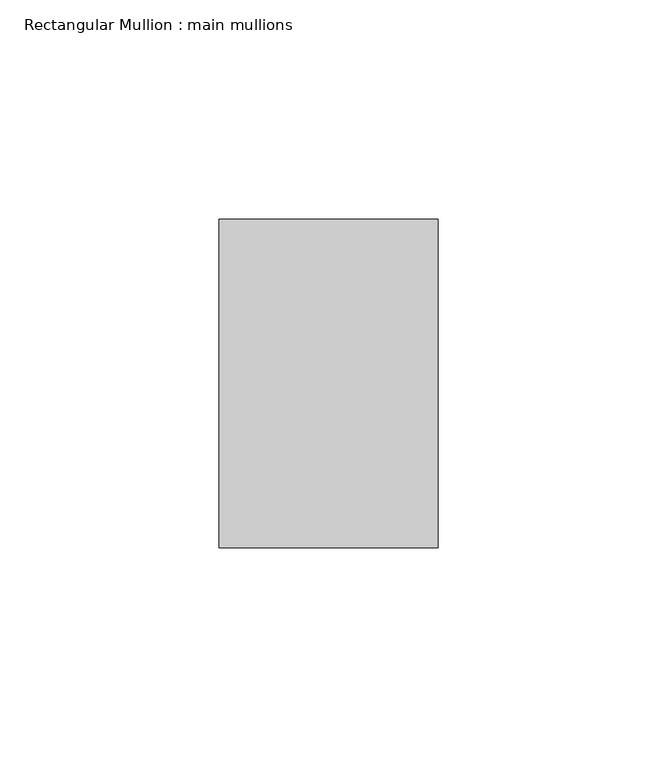
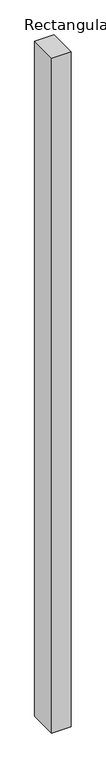
"""IFC4 building model written with IfcOpenShell, lengths in millimetres: member geometry, Rectangular Mullion : main mullions."""

from ifc_helpers import new_model, si_unit, frame, origin, place, context, project, spatial, polyline, outline, extrude, source, transform, mapped, element, save


def rectangular_mullion_main_mullions_97ba9194(model_context):
    return source(origin(), model_context, "Body", "SweptSolid", [
        extrude(outline(polyline([(25.0, 37.5), (25.0, -37.5), (-25.0, -37.5), (-25.0, 37.5), (25.0, 37.5)])), frame((0.0, 0.0, -1825.0), z_axis=(0.0, 0.0, 1.0), x_axis=(1.0, 0.0, 0.0)), (0.0, 0.0, 1.0), 1825.0),
    ])


if __name__ == "__main__":
    model = new_model("IFC4")
    model_context = context("Model", 3, world=origin())
    ifc_project = project(units=[si_unit("LENGTHUNIT", "METRE", prefix="MILLI")], contexts=[model_context])
    site = spatial("IfcSite", under=ifc_project)
    building = spatial("IfcBuilding", under=site)
    placement = place(None, origin())
    rectangular_mullion_main_mullions_shape = rectangular_mullion_main_mullions_97ba9194(model_context)
    element("IfcMember", 1, ObjectType="Rectangular Mullion : main mullions", at=placement, inside=building, context=model_context, shape_type="MappedRepresentation", body=[
        mapped(rectangular_mullion_main_mullions_shape, transform((0.0, 0.0, 0.0), x_axis=(1.0, 0.0, 0.0), y_axis=(0.0, 1.0, 0.0), z_axis=(0.0, 0.0, 1.0))),
    ])
    save(model, "model.ifc")

# Revit data of these elements
# Type "Rectangular Mullion : main mullions"
#   built-in parameter 1007304 = 0.246063 (stored number, unit not read)
#   built-in parameter 1007301 = 0.082021 (stored number, unit not read)
#   built-in parameter 1007300 = 0.082021 (stored number, unit not read)
# Element 1 (IfcMember, "Rectangular Mullion : main mullions")
#   Materials on its faces: "Aluminum"
# Materials
#   "Aluminum": class "Metal", colour RGB 136 136 136, transparency 0, Description = "Aluminum 6061", Cost = 0
